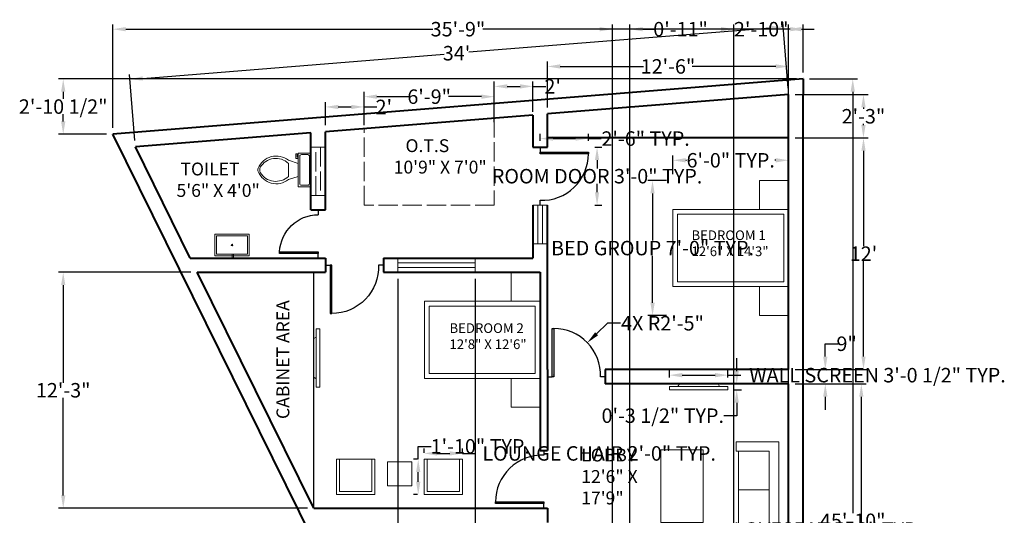
# Model space of a CAD drawing. Units: inches. Extents: x 927 to 1540, y 259 to 890.
# Tile 4 of 4: x 927 to 1540, y 582 to 890. Entities that reach past the tile are written whole.
import ezdxf

# ---------------------------------------------------------------- set-up
doc = ezdxf.new("R2010")
doc.units = ezdxf.units.IN
doc.header["$MEASUREMENT"] = 0
doc.linetypes.add('ACAD_ISO02W100', pattern=[15, 12, -3])
for name, color, linetype, lineweight in [('A-ANNO-DIMS', 2, 'Continuous', 18), ('A-AREA-IDEN', 7, 'Continuous', 25), ('A-DOOR', 3, 'Continuous', 25), ('A-EQPM', 8, 'Continuous', 18), ('A-FLOR-CASE', 9, 'Continuous', 25), ('A-FLOR-FIXT', 9, 'Continuous', 18), ('A-FLOR-OVHD', 8, 'ACAD_ISO02W100', 18), ('A-FURN', 8, 'Continuous', 18), ('A-GLAZ', 4, 'Continuous', 18), ('A-GLAZ-HIDN', 4, 'ACAD_ISO02W100', 18), ('A-WALL', 7, 'Continuous', 40)]:
    doc.layers.add(name, color=color, linetype=linetype, lineweight=lineweight)
doc.styles.get("Standard").update_dxf_attribs({"font": 'arial.ttf'})
doc.dimstyles.get("Standard").update_dxf_attribs({"dimtxt": 9, "dimasz": 8, "dimexe": 3, "dimexo": 4, "dimgap": 0.09, "dimtad": 0, "dimtih": 1, "dimtoh": 1, "dimdec": 0, "dimzin": 0, "dimdsep": 46, "dimlunit": 3, "dimtxsty": 'Standard', "dimcen": 0.09, "dimadec": 0, "dimazin": 0, "dimtfac": 1, "dimtdec": 0, "dimtofl": 0, "dimtmove": 0, "dimatfit": 3, "dimfxl": 1, "dimtolj": 1, "dimtzin": 0, "dimarcsym": 0})

# ---------------------------------------------------------------- blocks, each defined once
blk = doc.blocks.new('*D6')
at = {"layer": 'A-ANNO-DIMS', "color": 0, "lineweight": -2, "transparency": 16777216}
for p, q in [((1405.16, 847.38), (1401.86, 888.41)), ((1394.13, 884.78), (1206.71, 869.73)), ((1003.85, 853.44), (1191.26, 868.49)), ((998.93, 814.75), (995.63, 855.79))]:
    blk.add_line(p, q, dxfattribs=at)
at = {"layer": 'A-ANNO-DIMS', "color": 0, "lineweight": 100, "transparency": 16777216}
for points in [[(1394.02, 886.11), (1394.23, 883.45), (1402.1, 885.42)], [(1003.74, 854.77), (1003.96, 852.11), (995.87, 852.8)]]:
    blk.add_solid(points, dxfattribs=at)
at = {"layer": 'Defpoints', "color": 0, "lineweight": 100, "transparency": 16777216}
for p in [(1402.1, 885.42), (1405.48, 843.39), (999.25, 810.77)]:
    blk.add_point(p, dxfattribs=at)
at = {"layer": 'A-ANNO-DIMS', "color": 0, "transparency": 16777216, "insert": (1198.99, 869.11), "char_height": 9, "attachment_point": 5}
blk.add_mtext("\\A1;34'", dxfattribs=at)
blk = doc.blocks.new('*D11')
at = {"layer": 'A-ANNO-DIMS', "color": 0, "lineweight": -2, "transparency": 16777216}
for p, q in [((1409.48, 663.39), (1453.72, 663.39)), ((1450.72, 655.39), (1450.72, 561.58)), ((1450.72, 458.39), (1450.72, 552.21)), ((1418.48, 450.39), (1453.72, 450.39))]:
    blk.add_line(p, q, dxfattribs=at)
at = {"layer": 'A-ANNO-DIMS', "color": 0, "lineweight": 100, "transparency": 16777216}
for points in [[(1449.39, 655.39), (1452.05, 655.39), (1450.72, 663.39)], [(1449.39, 458.39), (1452.05, 458.39), (1450.72, 450.39)]]:
    blk.add_solid(points, dxfattribs=at)
at = {"layer": 'Defpoints', "color": 0, "lineweight": 100, "transparency": 16777216}
for p in [(1405.48, 663.39), (1450.72, 663.39), (1414.48, 450.39)]:
    blk.add_point(p, dxfattribs=at)
at = {"layer": 'A-ANNO-DIMS', "color": 0, "transparency": 16777216, "insert": (1450.72, 556.89), "char_height": 9, "attachment_point": 5}
blk.add_mtext('\\A1;17\'-9"', dxfattribs=at)
blk = doc.blocks.new('*D12')
at = {"layer": 'A-ANNO-DIMS', "color": 0, "lineweight": -2, "transparency": 16777216}
for p, q in [((1428.32, 680.39), (1428.32, 688.39)), ((1428.32, 688.39), (1436.32, 688.39)), ((1409.48, 672.39), (1431.32, 672.39)), ((1409.48, 663.39), (1431.32, 663.39)), ((1428.32, 655.39), (1428.32, 647.39))]:
    blk.add_line(p, q, dxfattribs=at)
at = {"layer": 'A-ANNO-DIMS', "color": 0, "lineweight": 100, "transparency": 16777216}
for points in [[(1426.98, 680.39), (1429.65, 680.39), (1428.32, 672.39)], [(1426.98, 655.39), (1429.65, 655.39), (1428.32, 663.39)]]:
    blk.add_solid(points, dxfattribs=at)
at = {"layer": 'Defpoints', "color": 0, "lineweight": 100, "transparency": 16777216}
for p in [(1405.48, 672.39), (1428.32, 672.39), (1405.48, 663.39)]:
    blk.add_point(p, dxfattribs=at)
at = {"layer": 'A-ANNO-DIMS', "color": 0, "transparency": 16777216, "insert": (1441.58, 688.39), "char_height": 9, "attachment_point": 5}
blk.add_mtext('\\A1;9"', dxfattribs=at)
blk = doc.blocks.new('*D13')
at = {"layer": 'A-ANNO-DIMS', "color": 0, "lineweight": -2, "transparency": 16777216}
for p, q in [((1409.48, 816.39), (1455.07, 816.39)), ((1452.07, 808.39), (1452.07, 749)), ((1452.07, 680.39), (1452.07, 739.78)), ((1409.48, 672.39), (1455.07, 672.39))]:
    blk.add_line(p, q, dxfattribs=at)
at = {"layer": 'A-ANNO-DIMS', "color": 0, "lineweight": 100, "transparency": 16777216}
for points in [[(1450.74, 808.39), (1453.4, 808.39), (1452.07, 816.39)], [(1450.74, 680.39), (1453.4, 680.39), (1452.07, 672.39)]]:
    blk.add_solid(points, dxfattribs=at)
at = {"layer": 'Defpoints', "color": 0, "lineweight": 100, "transparency": 16777216}
for p in [(1405.48, 816.39), (1452.07, 816.39), (1405.48, 672.39)]:
    blk.add_point(p, dxfattribs=at)
at = {"layer": 'A-ANNO-DIMS', "color": 0, "transparency": 16777216, "insert": (1452.07, 744.39), "char_height": 9, "attachment_point": 5}
blk.add_mtext("\\A1;12'", dxfattribs=at)
blk = doc.blocks.new('*D14')
at = {"layer": 'A-ANNO-DIMS', "color": 0, "lineweight": -2, "transparency": 16777216}
for p, q in [((1409.48, 843.39), (1455.04, 843.39)), ((1452.04, 835.39), (1452.04, 834.58)), ((1452.04, 824.39), (1452.04, 825.2)), ((1409.48, 816.39), (1455.04, 816.39))]:
    blk.add_line(p, q, dxfattribs=at)
at = {"layer": 'A-ANNO-DIMS', "color": 0, "lineweight": 100, "transparency": 16777216}
for points in [[(1450.71, 835.39), (1453.38, 835.39), (1452.04, 843.39)], [(1450.71, 824.39), (1453.38, 824.39), (1452.04, 816.39)]]:
    blk.add_solid(points, dxfattribs=at)
at = {"layer": 'Defpoints', "color": 0, "lineweight": 100, "transparency": 16777216}
for p in [(1405.48, 843.39), (1452.04, 843.39), (1405.48, 816.39)]:
    blk.add_point(p, dxfattribs=at)
at = {"layer": 'A-ANNO-DIMS', "color": 0, "transparency": 16777216, "insert": (1452.04, 829.89), "char_height": 9, "attachment_point": 5}
blk.add_mtext('\\A1;2\'-3"', dxfattribs=at)
blk = doc.blocks.new('*D16')
at = {"layer": 'A-ANNO-DIMS', "color": 0, "lineweight": -2, "transparency": 16777216}
for p, q in [((1255.48, 835.34), (1255.48, 863.88)), ((1405.48, 835.34), (1405.48, 863.88)), ((1263.48, 860.88), (1315.35, 860.88)), ((1397.48, 860.88), (1345.6, 860.88))]:
    blk.add_line(p, q, dxfattribs=at)
at = {"layer": 'A-ANNO-DIMS', "color": 0, "lineweight": 100, "transparency": 16777216}
for points in [[(1263.48, 862.21), (1263.48, 859.54), (1255.48, 860.88)], [(1397.48, 862.21), (1397.48, 859.54), (1405.48, 860.88)]]:
    blk.add_solid(points, dxfattribs=at)
at = {"layer": 'Defpoints', "color": 0, "lineweight": 100, "transparency": 16777216}
for p in [(1405.48, 860.88), (1255.48, 831.34), (1405.48, 831.34)]:
    blk.add_point(p, dxfattribs=at)
at = {"layer": 'A-ANNO-DIMS', "color": 0, "transparency": 16777216, "insert": (1330.48, 860.88), "char_height": 9, "attachment_point": 5}
blk.add_mtext('\\A1;12\'-6"', dxfattribs=at)
blk = doc.blocks.new('*D17')
at = {"layer": 'A-ANNO-DIMS', "color": 0, "lineweight": -2, "transparency": 16777216}
for p, q in [((1222.48, 832.69), (1222.48, 851.47)), ((1246.48, 832.69), (1246.48, 851.47)), ((1230.48, 848.47), (1238.48, 848.47)), ((1246.48, 848.47), (1254.48, 848.47))]:
    blk.add_line(p, q, dxfattribs=at)
at = {"layer": 'A-ANNO-DIMS', "color": 0, "lineweight": 100, "transparency": 16777216}
for points in [[(1230.48, 849.8), (1230.48, 847.13), (1222.48, 848.47)], [(1238.48, 849.8), (1238.48, 847.13), (1246.48, 848.47)]]:
    blk.add_solid(points, dxfattribs=at)
at = {"layer": 'Defpoints', "color": 0, "lineweight": 100, "transparency": 16777216}
for p in [(1246.48, 848.47), (1222.48, 828.69), (1246.48, 828.69)]:
    blk.add_point(p, dxfattribs=at)
at = {"layer": 'A-ANNO-DIMS', "color": 0, "transparency": 16777216, "insert": (1258.79, 848.47), "char_height": 9, "attachment_point": 5}
blk.add_mtext("\\A1;2'", dxfattribs=at)
blk = doc.blocks.new('*D18')
at = {"layer": 'A-ANNO-DIMS', "color": 0, "lineweight": -2, "transparency": 16777216}
for p, q in [((1141.48, 826.19), (1141.48, 845.08)), ((1222.48, 826.19), (1222.48, 845.08)), ((1149.48, 842.08), (1169.9, 842.08)), ((1214.48, 842.08), (1194.05, 842.08))]:
    blk.add_line(p, q, dxfattribs=at)
at = {"layer": 'A-ANNO-DIMS', "color": 0, "lineweight": 100, "transparency": 16777216}
for points in [[(1149.48, 843.41), (1149.48, 840.75), (1141.48, 842.08)], [(1214.48, 843.41), (1214.48, 840.75), (1222.48, 842.08)]]:
    blk.add_solid(points, dxfattribs=at)
at = {"layer": 'Defpoints', "color": 0, "lineweight": 100, "transparency": 16777216}
for p in [(1222.48, 842.08), (1141.48, 822.19), (1222.48, 822.19)]:
    blk.add_point(p, dxfattribs=at)
at = {"layer": 'A-ANNO-DIMS', "color": 0, "transparency": 16777216, "insert": (1181.98, 842.08), "char_height": 9, "attachment_point": 5}
blk.add_mtext('\\A1;6\'-9"', dxfattribs=at)
blk = doc.blocks.new('*D19')
at = {"layer": 'A-ANNO-DIMS', "color": 0, "lineweight": -2, "transparency": 16777216}
for p, q in [((1117.48, 824.26), (1117.48, 838.68)), ((1125.48, 835.68), (1133.48, 835.68)), ((1141.48, 824.26), (1141.48, 838.68)), ((1141.48, 835.68), (1149.48, 835.68))]:
    blk.add_line(p, q, dxfattribs=at)
at = {"layer": 'A-ANNO-DIMS', "color": 0, "lineweight": 100, "transparency": 16777216}
for points in [[(1125.48, 837.01), (1125.48, 834.34), (1117.48, 835.68)], [(1133.48, 837.01), (1133.48, 834.34), (1141.48, 835.68)]]:
    blk.add_solid(points, dxfattribs=at)
at = {"layer": 'Defpoints', "color": 0, "lineweight": 100, "transparency": 16777216}
for p in [(1141.48, 835.68), (1117.48, 820.26), (1141.48, 820.26)]:
    blk.add_point(p, dxfattribs=at)
at = {"layer": 'A-ANNO-DIMS', "color": 0, "transparency": 16777216, "insert": (1153.79, 835.68), "char_height": 9, "attachment_point": 5}
blk.add_mtext("\\A1;2'", dxfattribs=at)
blk = doc.blocks.new('DOOR-SINGLE-36-OPENING')
for p, q in [((3, 0), (3, 30)), ((3, 30), (4, 30)), ((4, 30), (4, 0)), ((0, 0), (3, 0)), ((4, 0), (3, 0)), ((36, 0), (33, 0))]:
    blk.add_line(p, q)
blk.add_arc((4, 0.98), 29.02, 358.05796, 90)
blk = doc.blocks.new('DOOR-SINGLE-30-OPENING')
for p, q in [((0, 24), (3, 24)), ((3, 24), (3, 0)), ((4, 24), (3, 24)), ((4, 0), (4, 24)), ((30, 24), (27, 24)), ((3, 0), (4, 0))]:
    blk.add_line(p, q)
blk.add_arc((2.98, 24), 24.02, 272.43775, 0)
blk = doc.blocks.new('SOFA-LOVESEAT-60')
for p, q in [((26.6182, 60.00004), (26.6182, 0)), ((0, 54.00004), (1.558, 54.00004)), ((1.558, 54.00004), (1.558, 6)), ((1.558, 54.00004), (20.6182, 53.99984)), ((20.6182, 53.99984), (20.6182, 6.00018)), ((1.558, 30.00004), (20.6182, 30.00004)), ((0, 6), (1.558, 6)), ((20.6182, 6.00018), (1.558, 6))]:
    blk.add_line(p, q)
for points in [[(0, 54.00004), (0, 60.00004), (26.6182, 60.00004)], [(26.6182, 0), (0, 0), (0, 6)]]:
    blk.add_lwpolyline(points)
blk = doc.blocks.new('BED-WITH-NIGHTSTANDS')
for points in [[(72, 84), (54, 84), (54, 66), (72, 66)], [(0, 66), (72, 66), (72, 18), (0, 18)], [(3, 63), (69, 63), (69, 21), (3, 21)], [(72, 18), (54, 18), (54, 0), (72, 0)]]:
    blk.add_lwpolyline(points, close=True)
blk = doc.blocks.new('LOUNGE-CHAIR-24')
for p, q in [((2, 22), (0, 22)), ((0, 0), (0, 22)), ((22, 22), (24, 22)), ((24, 22), (24, 0)), ((24, 0), (0, 0))]:
    blk.add_line(p, q)
blk.add_lwpolyline([(22, 2), (2, 2), (2, 22), (22, 22)], close=True)
blk = doc.blocks.new('SCREEN-WALL-MOUNT')
for p, q in [((0, 30.25), (1.49, 31.23)), ((0, 6.25), (1.49, 5.16))]:
    blk.add_line(p, q)
blk.add_lwpolyline([(1.49, 36.41), (3.73, 36.41), (3.73, 0), (1.49, 0)], close=True)
blk = doc.blocks.new('WC-TANK-TYPE')
for p, q in [((23.5, 17.5), (23.5, 20.5)), ((23.5, 20.5), (24.5, 20.5)), ((24.5, 20.5), (24.5, 18.5)), ((24.5, 18.5), (25, 18.5)), ((25, 14.5), (19, 16.5)), ((19, 6.5), (19, 14.5)), ((25, 17.5), (23.5, 17.5)), ((25, 6.5), (19, 4.5)), ((27, 1), (31, 1))]:
    blk.add_line(p, q)
blk.add_lwpolyline([(25, 0), (33, 0), (33, 21), (25, 21)], close=True)
for points in [[(26, 19), (26, 2)], [(31, 20), (27, 20)], [(32, 2), (32, 19)]]:
    blk.add_lwpolyline(points)
for centre, radius, start, end in [((11.42, 6.98), 12.17, 51.46911, 157.97143), ((26.87, 19.12), 0.884, 81.8699, 188.1301), ((31.12, 19.12), 0.884, 351.8699, 98.1301), ((11.18, 6.3), 11.33, 46.36773, 148.94682), ((4, 10.5), 4, 164.86053, 195.13947), ((11.42, 14.02), 12.17, 202.02843, 308.53071), ((5.12, 10.5), 4, 155.73182, 204.26817), ((11.18, 14.7), 11.33, 211.05301, 313.63209), ((26.87, 1.88), 0.884, 171.8699, 278.1301), ((31.12, 1.88), 0.884, 261.8699, 8.1301)]:
    blk.add_arc(centre, radius, start, end)
blk = doc.blocks.new('LAVATORY-RECTANGULAR')
for p, q in [((10.69, 2.5), (10.69, 0)), ((11.69, 2.5), (11.69, 0))]:
    blk.add_line(p, q)
for points in [[(0, 1.5), (21.39, 1.5), (21.39, 14.9), (0, 14.9)], [(1, 2.5), (20.39, 2.5), (20.39, 13.9), (1, 13.9)]]:
    blk.add_lwpolyline(points, close=True)
blk.add_circle((10.69, 8.2), 0.491)
blk = doc.blocks.new('*D32')
at = {"layer": 'A-ANNO-DIMS', "color": 0, "lineweight": -2, "transparency": 16777216}
for p, q in [((1284.98, 810.61), (1289.38, 810.61)), ((1286.38, 802.61), (1286.38, 797.36)), ((1286.38, 782.61), (1286.38, 787.86)), ((1284.98, 774.61), (1289.38, 774.61))]:
    blk.add_line(p, q, dxfattribs=at)
at = {"layer": 'A-ANNO-DIMS', "color": 0, "lineweight": 100, "transparency": 16777216}
for points in [[(1285.04, 802.61), (1287.71, 802.61), (1286.38, 810.61)], [(1285.04, 782.61), (1287.71, 782.61), (1286.38, 774.61)]]:
    blk.add_solid(points, dxfattribs=at)
at = {"layer": 'Defpoints', "color": 0, "lineweight": 100, "transparency": 16777216}
for p in [(1280.98, 810.61), (1280.98, 774.61), (1286.38, 774.61)]:
    blk.add_point(p, dxfattribs=at)
at = {"layer": 'A-ANNO-DIMS', "color": 0, "transparency": 16777216, "insert": (1286.38, 792.61), "char_height": 9, "attachment_point": 5}
blk.add_mtext('\\A1;ROOM DOOR 3\'-0" TYP.', dxfattribs=at)
blk = doc.blocks.new('*D33')
at = {"layer": 'A-ANNO-DIMS', "color": 0, "lineweight": -2, "transparency": 16777216}
for p, q in [((1250.98, 814.61), (1250.98, 819.01)), ((1258.98, 816.01), (1272.98, 816.01)), ((1280.98, 814.61), (1280.98, 819.01)), ((1280.98, 816.01), (1288.98, 816.01))]:
    blk.add_line(p, q, dxfattribs=at)
at = {"layer": 'A-ANNO-DIMS', "color": 0, "lineweight": 100, "transparency": 16777216}
for points in [[(1258.98, 817.35), (1258.98, 814.68), (1250.98, 816.01)], [(1272.98, 817.35), (1272.98, 814.68), (1280.98, 816.01)]]:
    blk.add_solid(points, dxfattribs=at)
at = {"layer": 'Defpoints', "color": 0, "lineweight": 100, "transparency": 16777216}
for p in [(1280.98, 816.01), (1250.98, 810.61), (1280.98, 810.61)]:
    blk.add_point(p, dxfattribs=at)
at = {"layer": 'A-ANNO-DIMS', "color": 0, "transparency": 16777216, "insert": (1316.57, 816.01), "char_height": 9, "attachment_point": 5}
blk.add_mtext('\\A1;2\'-6" TYP.', dxfattribs=at)
blk = doc.blocks.new('*D36')
at = {"layer": 'A-ANNO-DIMS', "color": 0, "lineweight": -2, "transparency": 16777216}
for p, q in [((1299.59, 567.82), (1299.59, 575.82)), ((1359.59, 567.82), (1359.59, 575.82)), ((1307.59, 572.82), (1351.59, 572.82)), ((1359.59, 572.82), (1367.59, 572.82))]:
    blk.add_line(p, q, dxfattribs=at)
at = {"layer": 'A-ANNO-DIMS', "color": 0, "lineweight": 100, "transparency": 16777216}
for points in [[(1307.59, 574.16), (1307.59, 571.49), (1299.59, 572.82)], [(1351.59, 574.16), (1351.59, 571.49), (1359.59, 572.82)]]:
    blk.add_solid(points, dxfattribs=at)
at = {"layer": 'Defpoints', "color": 0, "lineweight": 100, "transparency": 16777216}
for p in [(1359.59, 572.82), (1299.59, 563.82), (1359.59, 563.82)]:
    blk.add_point(p, dxfattribs=at)
at = {"layer": 'A-ANNO-DIMS', "color": 0, "transparency": 16777216, "insert": (1429.85, 572.82), "char_height": 9, "attachment_point": 5}
blk.add_mtext('\\A1;LOVESEAT 5\'-0" TYP.', dxfattribs=at)
blk = doc.blocks.new('*D38')
at = {"layer": 'A-ANNO-DIMS', "color": 0, "lineweight": -2, "transparency": 16777216}
for p, q in [((1329.48, 789.9), (1317.88, 789.9)), ((1320.88, 781.9), (1320.88, 752.65)), ((1320.88, 713.9), (1320.88, 743.16)), ((1329.48, 705.9), (1317.88, 705.9))]:
    blk.add_line(p, q, dxfattribs=at)
at = {"layer": 'A-ANNO-DIMS', "color": 0, "lineweight": 100, "transparency": 16777216}
for points in [[(1319.54, 781.9), (1322.21, 781.9), (1320.88, 789.9)], [(1319.54, 713.9), (1322.21, 713.9), (1320.88, 705.9)]]:
    blk.add_solid(points, dxfattribs=at)
at = {"layer": 'Defpoints', "color": 0, "lineweight": 100, "transparency": 16777216}
for p in [(1320.88, 789.9), (1333.48, 789.9), (1333.48, 705.9)]:
    blk.add_point(p, dxfattribs=at)
at = {"layer": 'A-ANNO-DIMS', "color": 0, "transparency": 16777216, "insert": (1320.88, 747.9), "char_height": 9, "attachment_point": 5}
blk.add_mtext('\\A1;BED GROUP 7\'-0" TYP.', dxfattribs=at)
blk = doc.blocks.new('*D39')
at = {"layer": 'A-ANNO-DIMS', "color": 0, "lineweight": -2, "transparency": 16777216}
for p, q in [((1333.48, 793.9), (1333.48, 805.5)), ((1341.48, 802.5), (1341.93, 802.5)), ((1397.48, 802.5), (1397.02, 802.5)), ((1405.48, 793.9), (1405.48, 805.5))]:
    blk.add_line(p, q, dxfattribs=at)
at = {"layer": 'A-ANNO-DIMS', "color": 0, "lineweight": 100, "transparency": 16777216}
for points in [[(1341.48, 803.84), (1341.48, 801.17), (1333.48, 802.5)], [(1397.48, 803.84), (1397.48, 801.17), (1405.48, 802.5)]]:
    blk.add_solid(points, dxfattribs=at)
at = {"layer": 'Defpoints', "color": 0, "lineweight": 100, "transparency": 16777216}
for p in [(1405.48, 802.5), (1333.48, 789.9), (1405.48, 789.9)]:
    blk.add_point(p, dxfattribs=at)
at = {"layer": 'A-ANNO-DIMS', "color": 0, "transparency": 16777216, "insert": (1369.48, 802.5), "char_height": 9, "attachment_point": 5}
blk.add_mtext('\\A1;6\'-0" TYP.', dxfattribs=at)
blk = doc.blocks.new('*D40')
at = {"layer": 'A-ANNO-DIMS', "color": 0, "lineweight": -2, "transparency": 16777216}
for p, q in [((1178.76, 620.59), (1178.76, 623.19)), ((1186.76, 620.19), (1194.76, 620.19)), ((1202.76, 620.59), (1202.76, 623.19)), ((1202.76, 620.19), (1210.76, 620.19))]:
    blk.add_line(p, q, dxfattribs=at)
at = {"layer": 'A-ANNO-DIMS', "color": 0, "lineweight": 100, "transparency": 16777216}
for points in [[(1186.76, 621.53), (1186.76, 618.86), (1178.76, 620.19)], [(1194.76, 621.53), (1194.76, 618.86), (1202.76, 620.19)]]:
    blk.add_solid(points, dxfattribs=at)
at = {"layer": 'Defpoints', "color": 0, "lineweight": 100, "transparency": 16777216}
for p in [(1202.76, 620.19), (1178.76, 616.59), (1202.76, 616.59)]:
    blk.add_point(p, dxfattribs=at)
at = {"layer": 'A-ANNO-DIMS', "color": 0, "transparency": 16777216, "insert": (1287.68, 620.19), "char_height": 9, "attachment_point": 5}
blk.add_mtext('\\A1;LOUNGE CHAIR 2\'-0" TYP.', dxfattribs=at)
blk = doc.blocks.new('*D41')
at = {"layer": 'A-ANNO-DIMS', "color": 0, "lineweight": -2, "transparency": 16777216}
for p, q in [((1175.16, 616.59), (1175.16, 624.59)), ((1175.16, 624.59), (1183.16, 624.59)), ((1174.76, 616.59), (1172.16, 616.59)), ((1175.16, 602.59), (1175.16, 608.59)), ((1174.76, 594.59), (1172.16, 594.59))]:
    blk.add_line(p, q, dxfattribs=at)
at = {"layer": 'A-ANNO-DIMS', "color": 0, "lineweight": 100, "transparency": 16777216}
for points in [[(1173.83, 608.59), (1176.49, 608.59), (1175.16, 616.59)], [(1173.83, 602.59), (1176.49, 602.59), (1175.16, 594.59)]]:
    blk.add_solid(points, dxfattribs=at)
at = {"layer": 'Defpoints', "color": 0, "lineweight": 100, "transparency": 16777216}
for p in [(1175.16, 616.59), (1178.76, 616.59), (1178.76, 594.59)]:
    blk.add_point(p, dxfattribs=at)
at = {"layer": 'A-ANNO-DIMS', "color": 0, "transparency": 16777216, "insert": (1213.75, 624.59), "char_height": 9, "attachment_point": 5}
blk.add_mtext('\\A1;1\'-10" TYP.', dxfattribs=at)
blk = doc.blocks.new('*D42')
at = {"layer": 'A-ANNO-DIMS', "color": 0, "lineweight": -2, "transparency": 16777216}
for p, q in [((1331.37, 667.39), (1331.37, 671.85)), ((1339.37, 668.85), (1359.78, 668.85)), ((1367.78, 667.39), (1367.78, 671.85)), ((1367.78, 668.85), (1375.78, 668.85))]:
    blk.add_line(p, q, dxfattribs=at)
at = {"layer": 'A-ANNO-DIMS', "color": 0, "lineweight": 100, "transparency": 16777216}
for points in [[(1339.37, 670.19), (1339.37, 667.52), (1331.37, 668.85)], [(1359.78, 670.19), (1359.78, 667.52), (1367.78, 668.85)]]:
    blk.add_solid(points, dxfattribs=at)
at = {"layer": 'Defpoints', "color": 0, "lineweight": 100, "transparency": 16777216}
for p in [(1367.78, 668.85), (1331.37, 663.39), (1367.78, 663.39)]:
    blk.add_point(p, dxfattribs=at)
at = {"layer": 'A-ANNO-DIMS', "color": 0, "transparency": 16777216, "insert": (1460.78, 668.85), "char_height": 9, "attachment_point": 5}
blk.add_mtext('\\A1;WALL SCREEN 3\'-0 1/2" TYP.', dxfattribs=at)
blk = doc.blocks.new('*D43')
at = {"layer": 'A-ANNO-DIMS', "color": 0, "lineweight": -2, "transparency": 16777216}
for p, q in [((1373.24, 671.39), (1373.24, 679.39)), ((1371.78, 663.39), (1376.24, 663.39)), ((1371.78, 659.66), (1376.24, 659.66)), ((1373.24, 651.66), (1373.24, 643.66)), ((1373.24, 643.66), (1365.24, 643.66))]:
    blk.add_line(p, q, dxfattribs=at)
at = {"layer": 'A-ANNO-DIMS', "color": 0, "lineweight": 100, "transparency": 16777216}
for points in [[(1371.91, 671.39), (1374.57, 671.39), (1373.24, 663.39)], [(1371.91, 651.66), (1374.57, 651.66), (1373.24, 659.66)]]:
    blk.add_solid(points, dxfattribs=at)
at = {"layer": 'Defpoints', "color": 0, "lineweight": 100, "transparency": 16777216}
for p in [(1367.78, 663.39), (1367.78, 659.66), (1373.24, 659.66)]:
    blk.add_point(p, dxfattribs=at)
at = {"layer": 'A-ANNO-DIMS', "color": 0, "transparency": 16777216, "insert": (1327.24, 643.66), "char_height": 9, "attachment_point": 5}
blk.add_mtext('\\A1;0\'-3 1/2" TYP.', dxfattribs=at)
blk = doc.blocks.new('*D50')
at = {"layer": 'A-ANNO-DIMS', "color": 0, "lineweight": -2, "transparency": 16777216}
for p, q in [((985.3, 822.67), (985.3, 887.04)), ((993.3, 884.04), (1184.35, 884.04)), ((1406.48, 884.04), (1215.44, 884.04)), ((1414.48, 857.14), (1414.48, 887.04))]:
    blk.add_line(p, q, dxfattribs=at)
at = {"layer": 'A-ANNO-DIMS', "color": 0, "lineweight": 100, "transparency": 16777216}
for points in [[(993.3, 885.38), (993.3, 882.71), (985.3, 884.04)], [(1406.48, 885.38), (1406.48, 882.71), (1414.48, 884.04)]]:
    blk.add_solid(points, dxfattribs=at)
at = {"layer": 'Defpoints', "color": 0, "lineweight": 100, "transparency": 16777216}
for p in [(1414.48, 884.04), (1414.48, 853.14), (985.3, 818.67)]:
    blk.add_point(p, dxfattribs=at)
at = {"layer": 'A-ANNO-DIMS', "color": 0, "transparency": 16777216, "insert": (1199.89, 884.04), "char_height": 9, "attachment_point": 5}
blk.add_mtext('\\A1;35\'-9"', dxfattribs=at)
blk = doc.blocks.new('*D51')
at = {"layer": 'A-ANNO-DIMS', "color": 0, "lineweight": -2, "transparency": 16777216}
for p, q in [((1418.48, 853.14), (1448.38, 853.14)), ((1445.38, 845.14), (1445.38, 582.95)), ((1445.38, 311.39), (1445.38, 573.58)), ((1418.48, 303.39), (1448.38, 303.39))]:
    blk.add_line(p, q, dxfattribs=at)
at = {"layer": 'A-ANNO-DIMS', "color": 0, "lineweight": 100, "transparency": 16777216}
for points in [[(1444.04, 845.14), (1446.71, 845.14), (1445.38, 853.14)], [(1444.04, 311.39), (1446.71, 311.39), (1445.38, 303.39)]]:
    blk.add_solid(points, dxfattribs=at)
at = {"layer": 'Defpoints', "color": 0, "lineweight": 100, "transparency": 16777216}
for p in [(1414.48, 853.14), (1445.38, 853.14), (1414.48, 303.39)]:
    blk.add_point(p, dxfattribs=at)
at = {"layer": 'A-ANNO-DIMS', "color": 0, "transparency": 16777216, "insert": (1445.38, 578.27), "char_height": 9, "attachment_point": 5}
blk.add_mtext('\\A1;45\'-10"', dxfattribs=at)
blk = doc.blocks.new('*D53')
at = {"layer": 'A-ANNO-DIMS', "color": 0, "lineweight": -2, "transparency": 16777216}
for p, q in [((1410.48, 853.14), (951.4, 853.14)), ((954.4, 845.14), (954.4, 840.65)), ((954.4, 826.67), (954.4, 831.17)), ((981.3, 818.67), (951.4, 818.67))]:
    blk.add_line(p, q, dxfattribs=at)
at = {"layer": 'A-ANNO-DIMS', "color": 0, "lineweight": 100, "transparency": 16777216}
for points in [[(953.07, 845.14), (955.74, 845.14), (954.4, 853.14)], [(953.07, 826.67), (955.74, 826.67), (954.4, 818.67)]]:
    blk.add_solid(points, dxfattribs=at)
at = {"layer": 'Defpoints', "color": 0, "lineweight": 100, "transparency": 16777216}
for p in [(954.4, 853.14), (1414.48, 853.14), (985.3, 818.67)]:
    blk.add_point(p, dxfattribs=at)
at = {"layer": 'A-ANNO-DIMS', "color": 0, "transparency": 16777216, "insert": (954.4, 835.91), "char_height": 9, "attachment_point": 5}
blk.add_mtext('\\A1;2\'-10 1/2"', dxfattribs=at)
blk = doc.blocks.new('*D54')
at = {"layer": 'A-ANNO-DIMS', "color": 0, "lineweight": -2, "transparency": 16777216}
for p, q in [((1363.48, 884.04), (1355.48, 884.04)), ((1371.48, 411.39), (1371.48, 887.04)), ((1405.48, 411.39), (1405.48, 887.04)), ((1413.48, 884.04), (1421.48, 884.04))]:
    blk.add_line(p, q, dxfattribs=at)
at = {"layer": 'A-ANNO-DIMS', "color": 0, "lineweight": 100, "transparency": 16777216}
for points in [[(1363.48, 885.38), (1363.48, 882.71), (1371.48, 884.04)], [(1413.48, 885.38), (1413.48, 882.71), (1405.48, 884.04)]]:
    blk.add_solid(points, dxfattribs=at)
at = {"layer": 'Defpoints', "color": 0, "lineweight": 100, "transparency": 16777216}
for p in [(1405.48, 884.04), (1371.48, 407.39), (1405.48, 407.39)]:
    blk.add_point(p, dxfattribs=at)
at = {"layer": 'A-ANNO-DIMS', "color": 0, "transparency": 16777216, "insert": (1388.48, 884.04), "char_height": 9, "attachment_point": 5}
blk.add_mtext('\\A1;2\'-10"', dxfattribs=at)
blk = doc.blocks.new('*D55')
at = {"layer": 'A-ANNO-DIMS', "color": 0, "lineweight": -2, "transparency": 16777216}
for p, q in [((1287.98, 884.04), (1279.98, 884.04)), ((1295.98, 445.39), (1295.98, 887.04)), ((1306.76, 445.39), (1306.76, 887.04)), ((1314.76, 884.04), (1322.76, 884.04))]:
    blk.add_line(p, q, dxfattribs=at)
at = {"layer": 'A-ANNO-DIMS', "color": 0, "lineweight": 100, "transparency": 16777216}
for points in [[(1287.98, 885.38), (1287.98, 882.71), (1295.98, 884.04)], [(1314.76, 885.38), (1314.76, 882.71), (1306.76, 884.04)]]:
    blk.add_solid(points, dxfattribs=at)
at = {"layer": 'Defpoints', "color": 0, "lineweight": 100, "transparency": 16777216}
for p in [(1306.76, 884.04), (1295.98, 441.39), (1306.76, 441.39)]:
    blk.add_point(p, dxfattribs=at)
at = {"layer": 'A-ANNO-DIMS', "color": 0, "transparency": 16777216, "insert": (1338.31, 884.04), "char_height": 9, "attachment_point": 5}
blk.add_mtext('\\A1;0\'-11"', dxfattribs=at)
blk = doc.blocks.new('*D56')
at = {"layer": 'A-ANNO-DIMS', "color": 0, "lineweight": -2, "transparency": 16777216}
for p, q in [((1033.74, 732.87), (951.4, 732.87)), ((954.4, 724.87), (954.4, 664.15)), ((954.4, 594.06), (954.4, 654.78)), ((1106.27, 586.06), (951.4, 586.06))]:
    blk.add_line(p, q, dxfattribs=at)
at = {"layer": 'A-ANNO-DIMS', "color": 0, "lineweight": 100, "transparency": 16777216}
for points in [[(953.07, 724.87), (955.74, 724.87), (954.4, 732.87)], [(953.07, 594.06), (955.74, 594.06), (954.4, 586.06)]]:
    blk.add_solid(points, dxfattribs=at)
at = {"layer": 'Defpoints', "color": 0, "lineweight": 100, "transparency": 16777216}
for p in [(954.4, 732.87), (1037.74, 732.87), (1110.27, 586.06)]:
    blk.add_point(p, dxfattribs=at)
at = {"layer": 'A-ANNO-DIMS', "color": 0, "transparency": 16777216, "insert": (954.4, 659.47), "char_height": 9, "attachment_point": 5}
blk.add_mtext('\\A1;12\'-3"', dxfattribs=at)
blk = doc.blocks.new('*D58')
at = {"layer": 'A-ANNO-DIMS', "color": 0, "lineweight": -2, "transparency": 16777216}
for p, q in [((1162.48, 728.87), (1162.48, 269.49)), ((1210.48, 728.87), (1210.48, 269.49)), ((1170.48, 272.49), (1174.24, 272.49)), ((1202.48, 272.49), (1198.71, 272.49))]:
    blk.add_line(p, q, dxfattribs=at)
at = {"layer": 'A-ANNO-DIMS', "color": 0, "lineweight": 100, "transparency": 16777216}
for points in [[(1170.48, 273.82), (1170.48, 271.16), (1162.48, 272.49)], [(1202.48, 273.82), (1202.48, 271.16), (1210.48, 272.49)]]:
    blk.add_solid(points, dxfattribs=at)
at = {"layer": 'Defpoints', "color": 0, "lineweight": 100, "transparency": 16777216}
for p in [(1162.48, 732.87), (1210.48, 732.87), (1210.48, 272.49)]:
    blk.add_point(p, dxfattribs=at)
at = {"layer": 'A-ANNO-DIMS', "color": 0, "transparency": 16777216, "insert": (1186.48, 272.49), "char_height": 9, "attachment_point": 5}
blk.add_mtext('\\A1;4\'-0"', dxfattribs=at)
blk = doc.blocks.new('*D59')
at = {"layer": 'A-ANNO-DIMS', "color": 0, "lineweight": -2, "transparency": 16777216}
for p, q in [((1292.86, 701.14), (1286.09, 694.6)), ((1300.86, 701.14), (1292.86, 701.14)), ((1259.39, 668.87), (1259.57, 668.87)), ((1259.48, 668.78), (1259.48, 668.96))]:
    blk.add_line(p, q, dxfattribs=at)
at = {"layer": 'A-ANNO-DIMS', "color": 0, "lineweight": 100, "transparency": 16777216}
blk.add_solid([(1285.17, 695.56), (1287.02, 693.64), (1280.34, 689.04)], dxfattribs=at)
at = {"layer": 'Defpoints', "color": 0, "lineweight": 100, "transparency": 16777216}
for p in [(1280.34, 689.04), (1259.48, 668.87)]:
    blk.add_point(p, dxfattribs=at)
at = {"layer": 'A-ANNO-DIMS', "color": 0, "transparency": 16777216, "insert": (1327.07, 701.14), "char_height": 9, "attachment_point": 5}
blk.add_mtext('\\A1;4X R2\'-5"', dxfattribs=at)

msp = doc.modelspace()

# ---------------------------------------------------------------- linework, layer by layer
at = {"layer": 'A-FLOR-CASE'}
msp.add_line((1110.27, 586.06), (1110.27, 732.87), dxfattribs=at)
at = {"layer": 'A-FLOR-OVHD'}
for p, q in [((1222.48, 828.69), (1222.48, 774.61)), ((1141.48, 774.61), (1141.48, 822.19)), ((1222.48, 774.61), (1141.48, 774.61))]:
    msp.add_line(p, q, dxfattribs=at)
at = {"layer": 'A-FURN'}
for points in [[(1352.35, 577.18), (1326.12, 577.18), (1326.12, 622.34), (1352.35, 622.34)], [(1156.12, 614.99), (1171.12, 614.99), (1171.12, 599.99), (1156.12, 599.99)]]:
    msp.add_lwpolyline(points, close=True, dxfattribs=at)
at = {"layer": 'A-GLAZ'}
for p, q in [((1108.48, 810.61), (1117.48, 810.61)), ((1117.48, 810.61), (1114.48, 810.61)), ((1108.48, 780.61), (1117.48, 780.61)), ((1114.48, 780.61), (1111.48, 780.61)), ((1246.48, 774.61), (1255.48, 774.61)), ((1249.48, 750.61), (1249.48, 774.61)), ((1252.48, 750.61), (1252.48, 774.61)), ((1246.48, 750.61), (1255.48, 750.61)), ((1162.48, 741.61), (1162.48, 732.87)), ((1210.48, 741.61), (1210.48, 732.87)), ((1162.48, 738.74), (1210.48, 738.74)), ((1162.48, 735.74), (1210.48, 735.74))]:
    msp.add_line(p, q, dxfattribs=at)
at = {"layer": 'A-GLAZ-HIDN'}
for p, q in [((1111.48, 780.61), (1111.48, 810.61)), ((1114.48, 810.61), (1114.48, 780.61))]:
    msp.add_line(p, q, dxfattribs=at)
at = {"layer": 'A-WALL'}
for p, q in [((1414.48, 853.14), (985.3, 818.67)), ((1414.48, 853.14), (1414.48, 843.39)), ((1405.48, 843.39), (1255.48, 831.34)), ((1405.48, 816.39), (1405.48, 843.39)), ((1414.48, 816.39), (1414.48, 843.39)), ((1246.48, 830.62), (1117.48, 820.26)), ((1246.48, 830.62), (1246.48, 810.61)), ((1255.48, 810.61), (1255.48, 831.34)), ((1239.89, 303.39), (985.3, 818.67)), ((1108.48, 819.54), (999.25, 810.77)), ((1108.48, 771.61), (1108.48, 819.54)), ((1117.48, 771.61), (1117.48, 820.26)), ((1405.48, 816.39), (1255.48, 816.39)), ((1405.48, 672.39), (1405.48, 816.39)), ((1414.48, 672.39), (1414.48, 816.39)), ((1033.42, 741.61), (999.25, 810.77)), ((1246.48, 810.61), (1255.48, 810.61)), ((1108.48, 771.61), (1117.48, 771.61)), ((1246.48, 774.61), (1246.48, 741.61)), ((1255.48, 672.39), (1255.48, 774.61)), ((1033.42, 741.61), (1108.48, 741.61)), ((1108.48, 741.61), (1117.48, 741.61)), ((1117.48, 741.61), (1117.48, 732.87)), ((1153.48, 741.61), (1246.48, 741.61)), ((1153.48, 741.61), (1153.48, 732.87)), ((1037.74, 732.87), (1117.48, 732.87)), ((1110.27, 586.06), (1037.74, 732.87)), ((1153.48, 732.87), (1250.98, 732.87)), ((1250.98, 732.87), (1250.98, 622.06)), ((1255.48, 672.39), (1255.48, 663.39)), ((1405.48, 672.39), (1291.48, 672.39)), ((1291.48, 672.39), (1291.48, 663.39)), ((1414.48, 663.39), (1414.48, 672.39)), ((1255.48, 663.39), (1255.48, 622.06)), ((1405.48, 663.39), (1291.48, 663.39)), ((1405.48, 450.39), (1405.48, 663.39)), ((1414.48, 450.39), (1414.48, 663.39)), ((1250.98, 622.06), (1255.48, 622.06)), ((1110.27, 586.06), (1255.48, 586.06)), ((1255.48, 586.06), (1255.48, 577.32))]:
    msp.add_line(p, q, dxfattribs=at)

# ---------------------------------------------------------------- block references
at = {"layer": 'A-DOOR'}
for p, rotation in [((1250.98, 810.61), 270), ((1253.23, 586.06), 89.99999999999991)]:
    msp.add_blockref('DOOR-SINGLE-36-OPENING', p, dxfattribs=dict(at, rotation=rotation))
at = {"layer": 'A-DOOR', "extrusion": (0, 0, -1), "zscale": -1}
for name, p, rotation in [('DOOR-SINGLE-30-OPENING', (-1088.98, 741.61), 90), ('DOOR-SINGLE-36-OPENING', (-1117.48, 737.24), 180)]:
    msp.add_blockref(name, p, dxfattribs=dict(at, rotation=rotation))
at = {"layer": 'A-DOOR'}
msp.add_blockref('DOOR-SINGLE-36-OPENING', (1255.48, 667.89), dxfattribs=at)
at = {"layer": 'A-EQPM'}
msp.add_blockref('SCREEN-WALL-MOUNT', (1110.27, 661.35), dxfattribs=at)
at = {"layer": 'A-EQPM', "rotation": 269.9999999999998}
msp.add_blockref('SCREEN-WALL-MOUNT', (1331.37, 663.39), dxfattribs=at)
at = {"layer": 'A-FLOR-FIXT'}
for name, p in [('WC-TANK-TYPE', (1075.48, 786.02)), ('LAVATORY-RECTANGULAR', (1048.68, 741.61))]:
    msp.add_blockref(name, p, dxfattribs=at)
at = {"layer": 'A-FURN'}
for name, p in [('BED-WITH-NIGHTSTANDS', (1333.48, 705.9)), ('BED-WITH-NIGHTSTANDS', (1178.98, 648.87)), ('SOFA-LOVESEAT-60', (1372.84, 567.49)), ('LOUNGE-CHAIR-24', (1178.76, 594.59))]:
    msp.add_blockref(name, p, dxfattribs=at)
at = {"layer": 'A-FURN', "extrusion": (0, 0, -1), "zscale": -1}
msp.add_blockref('LOUNGE-CHAIR-24', (-1148.27, 594.59), dxfattribs=at)

# ---------------------------------------------------------------- texts
at = {"layer": 'A-AREA-IDEN', "attachment_point": 1}
for s, insert, char_height in [('   O.T.S \\P10\'9" X 7\'0"', (1159.91, 815.59), 8), (' TOILET \\P5\'6" X 4\'0"', (1024.87, 801.08), 8), ('BEDROOM 1\\P12\'6" X 14\'3"', (1345.11, 758.89), 6), ('BEDROOM 2\\P12\'8" X 12\'6"', (1194.62, 701.11), 6), ('LOBBY\\P12\'6" X \\P17\'9"', (1276.54, 623.16), 8)]:
    msp.add_mtext_dynamic_manual_height_columns(s, width=78.5806, gutter_width=1, heights=[0], dxfattribs=dict(at, insert=insert, char_height=char_height))
at = {"layer": 'A-AREA-IDEN', "insert": (1087.02, 641.58), "char_height": 8, "attachment_point": 1, "rotation": 90}
msp.add_mtext_dynamic_manual_height_columns('CABINET AREA', width=83.9619, gutter_width=1, heights=[0], dxfattribs=at)

# ---------------------------------------------------------------- dimensions: what is measured, and where the dimension line sits
at = {"layer": 'A-ANNO-DIMS'}
for base, p1, p2, override, picture, middle in [((1414.48, 884.04), (985.3, 818.67), (1414.48, 853.14), {"dimdec": 1, "dimlfac": 1, "dimrnd": 0, "dimzin": 1, "dimdsep": 46, "dimlunit": 4, "dimfrac": 2}, '*D50', (1199.89, 884.04)), ((1306.76, 884.04), (1295.98, 441.39), (1306.76, 441.39), {"dimdec": 1, "dimlfac": 1, "dimrnd": 0, "dimzin": 1, "dimdsep": 46, "dimlunit": 4, "dimfrac": 2}, '*D55', (1338.31, 884.04)), ((1405.48, 884.04), (1371.48, 407.39), (1405.48, 407.39), {"dimdec": 1, "dimlfac": 1, "dimrnd": 0, "dimzin": 1, "dimdsep": 46, "dimlunit": 4, "dimfrac": 2}, '*D54', (1388.48, 884.04)), ((1405.48, 860.88), (1255.48, 831.34), (1405.48, 831.34), {"dimclrd": 0, "dimclre": 0, "dimclrt": 0}, '*D16', (1330.48, 860.88)), ((1246.48, 848.47), (1222.48, 828.69), (1246.48, 828.69), {"dimclrd": 0, "dimclre": 0, "dimclrt": 0}, '*D17', (1258.79, 848.47)), ((1222.48, 842.08), (1141.48, 822.19), (1222.48, 822.19), {"dimclrd": 0, "dimclre": 0, "dimclrt": 0}, '*D18', (1181.98, 842.08)), ((1141.48, 835.68), (1117.48, 820.26), (1141.48, 820.26), {"dimclrd": 0, "dimclre": 0, "dimclrt": 0}, '*D19', (1153.79, 835.68)), ((1210.48, 272.49), (1162.48, 732.87), (1210.48, 732.87), {"dimdec": 1, "dimlfac": 1, "dimrnd": 0, "dimzin": 1, "dimdsep": 46, "dimlunit": 4, "dimfrac": 2}, '*D58', (1186.48, 272.49))]:
    dim = msp.add_linear_dim(base=base, p1=p1, p2=p2, dimstyle='Standard', override=override, dxfattribs=at)
    dim.commit()
    dim.dimension.update_dxf_attribs({"geometry": picture, "text_midpoint": middle})
dim = msp.add_aligned_dim(p1=(999.25, 810.77), p2=(1405.48, 843.39), distance=42.17, dimstyle='Standard', override={"dimclrd": 0, "dimclre": 0, "dimclrt": 0}, dxfattribs=at)
dim.commit()
dim.dimension.update_dxf_attribs({"geometry": '*D6', "text_midpoint": (1198.99, 869.11)})
for base, p1, p2, override, picture, middle in [((954.4, 853.14), (985.3, 818.67), (1414.48, 853.14), {"dimdec": 1, "dimlfac": 1, "dimrnd": 0, "dimzin": 1, "dimdsep": 46, "dimlunit": 4, "dimfrac": 2}, '*D53', (954.4, 835.91)), ((1445.3775, 853.1431), (1414.4775, 303.3913), (1414.4775, 853.1431), {"dimdec": 1, "dimlfac": 1, "dimrnd": 0, "dimzin": 1, "dimdsep": 46, "dimlunit": 4, "dimfrac": 2}, '*D51', (1445.3775, 578.2672)), ((1452.04, 843.39), (1405.48, 816.39), (1405.48, 843.39), {"dimclrd": 0, "dimclre": 0, "dimclrt": 0}, '*D14', (1452.04, 829.89)), ((1452.07, 816.39), (1405.48, 672.39), (1405.48, 816.39), {"dimclrd": 0, "dimclre": 0, "dimclrt": 0}, '*D13', (1452.07, 744.39)), ((954.4, 732.87), (1110.27, 586.06), (1037.74, 732.87), {"dimdec": 1, "dimlfac": 1, "dimrnd": 0, "dimzin": 1, "dimdsep": 46, "dimlunit": 4, "dimfrac": 2}, '*D56', (954.4, 659.47)), ((1428.32, 672.39), (1405.48, 663.39), (1405.48, 672.39), {"dimclrd": 0, "dimclre": 0, "dimclrt": 0}, '*D12', (1441.58, 688.39)), ((1450.72, 663.39), (1414.48, 450.39), (1405.48, 663.39), {"dimclrd": 0, "dimclre": 0, "dimclrt": 0}, '*D11', (1450.72, 556.89))]:
    dim = msp.add_linear_dim(base=base, p1=p1, p2=p2, angle=90, dimstyle='Standard', override=override, dxfattribs=at)
    dim.commit()
    dim.dimension.update_dxf_attribs({"geometry": picture, "text_midpoint": middle})
for base, p1, p2, text, picture, middle in [((1280.98, 816.01), (1250.98, 810.61), (1280.98, 810.61), '<> TYP.', '*D33', (1316.57, 816.01)), ((1405.48, 802.5), (1333.48, 789.9), (1405.48, 789.9), '<> TYP.', '*D39', (1369.48, 802.5)), ((1367.78, 668.85), (1331.37, 663.39), (1367.78, 663.39), 'WALL SCREEN <> TYP.', '*D42', (1460.78, 668.85)), ((1202.76, 620.19), (1178.76, 616.59), (1202.76, 616.59), 'LOUNGE CHAIR <> TYP.', '*D40', (1287.68, 620.19)), ((1359.59, 572.82), (1299.59, 563.82), (1359.59, 563.82), 'LOVESEAT <> TYP.', '*D36', (1429.85, 572.82))]:
    dim = msp.add_linear_dim(base=base, p1=p1, p2=p2, text=text, dimstyle='Standard', override={"dimdec": 1, "dimlfac": 1, "dimrnd": 0, "dimzin": 1, "dimdsep": 46, "dimlunit": 4, "dimfrac": 2}, dxfattribs=at)
    dim.commit()
    dim.dimension.update_dxf_attribs({"geometry": picture, "text_midpoint": middle})
for base, p1, p2, angle, text, picture, middle in [((1286.38, 774.61), (1280.98, 810.61), (1280.98, 774.61), 270, 'ROOM DOOR <> TYP.', '*D32', (1286.38, 792.61)), ((1320.88, 789.9), (1333.48, 705.9), (1333.48, 789.9), 90, 'BED GROUP <> TYP.', '*D38', (1320.88, 747.9)), ((1373.24, 659.66), (1367.78, 663.39), (1367.78, 659.66), 270, '<> TYP.', '*D43', (1327.24, 643.66)), ((1175.16, 616.59), (1178.76, 594.59), (1178.76, 616.59), 90, '<> TYP.', '*D41', (1213.75, 624.59))]:
    dim = msp.add_linear_dim(base=base, p1=p1, p2=p2, angle=angle, text=text, dimstyle='Standard', override={"dimdec": 1, "dimlfac": 1, "dimrnd": 0, "dimzin": 1, "dimdsep": 46, "dimlunit": 4, "dimfrac": 2}, dxfattribs=at)
    dim.commit()
    dim.dimension.update_dxf_attribs({"geometry": picture, "text_midpoint": middle})
dim = msp.add_radius_dim(center=(1259.48, 668.87), mpoint=(1280.34, 689.04), text='4X <>', dimstyle='Standard', override={"dimdec": 1, "dimlfac": 1, "dimrnd": 0, "dimzin": 1, "dimdsep": 46, "dimlunit": 4, "dimfrac": 2}, dxfattribs=at)
dim.commit()
dim.dimension.update_dxf_attribs({"geometry": '*D59', "text_midpoint": (1327.07, 701.14), "dimtype": 164})

doc.saveas('drawing.dxf')
